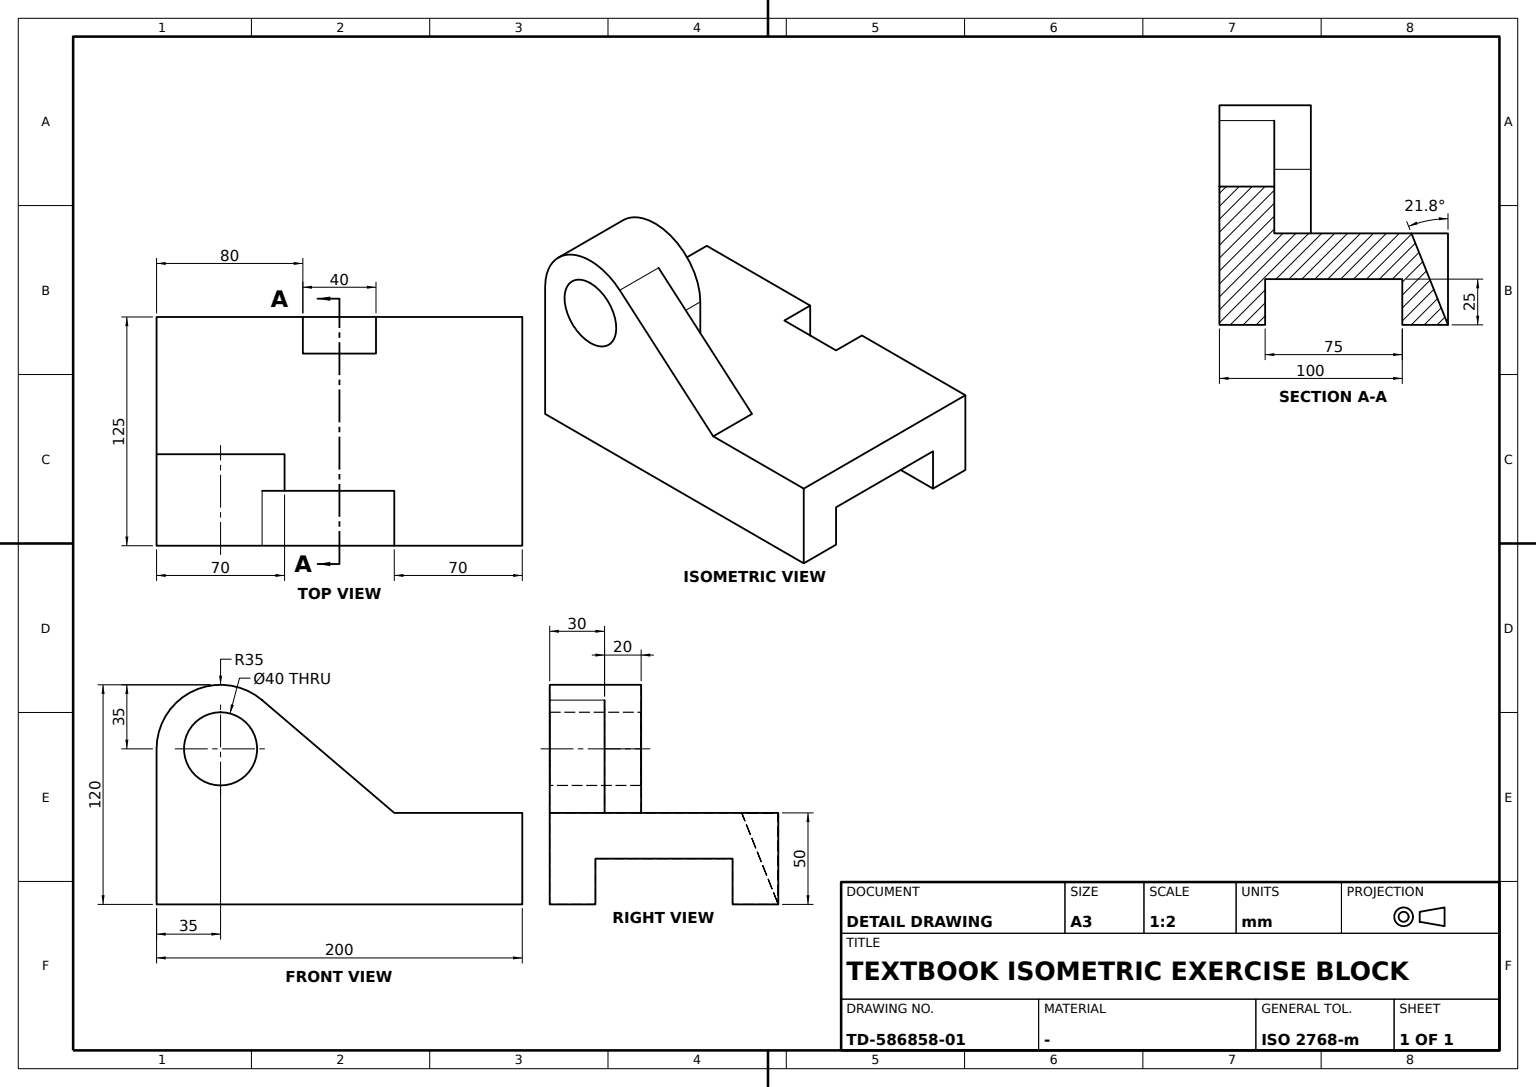
CATIA V5 part; units mm, degrees
sketch "Sketch1" plane through (0, 0, 0) normal (1, 0, 0) x (0, 1, 0)
  line L0 (-62.5, 50) -> (62.5, 50)
  line L1 (62.5, 50) -> (62.5, 0)
  point P0 (62.5, 0)
  line L2 (62.5, 0) -> (37.5, 0)
  line L3 (37.5, 0) -> (37.5, 25)
  line L4 (37.5, 25) -> (-37.5, 25)
  line L5 (-37.5, 25) -> (-37.5, 0)
  point P1 (-37.5, 0)
  line L6 (-37.5, 0) -> (-62.5, 0)
  line L7 (-62.5, 0) -> (-62.5, 50)
  dimension "length L4" = 75
  dimension "length L0" = 125
  dimension "length L5" = 25
  dimension "length L7" = 50
  constraint horizontal L0 x-axis
  constraint horizontal L2 x-axis
  constraint horizontal L4 x-axis
  constraint horizontal L6 x-axis
  constraint coincidence P0 x-axis
  constraint coincidence P1 x-axis
  constraint vertical L1 y-axis
  constraint vertical L3 y-axis
  constraint vertical L5 y-axis
  constraint vertical L7 y-axis
  constraint symmetry L7 L1 y-axis
  constraint symmetry L5 L3 y-axis
extrude "Pad1" add sketch "Sketch1" along normal mid plane 200
sketch "Sketch2" plane through (0, 0, 0) normal (1, 0, 0) x (0, 1, 0)
  line L0 (42.5, 50) -> (62.5, 0)
  point P0 (62.5, 0)
  line L1 (62.5, 0) -> (62.5, 50)
  line L2 (62.5, 50) -> (42.5, 50)
  line L3 (62.5, 0) -> (62.5, 50) construction
  line L4 (62.5, 50) -> (-62.5, 50) construction
  dimension "length L2" = 20
  dimension "distance L1 L3" = 0
  dimension "distance L2 L4" = 0
  constraint coincidence P0 x-axis
  constraint vertical L1 y-axis
  constraint horizontal L2 x-axis
extrude "Pocket1" cut sketch "Sketch2" along normal mid plane 40
sketch "Sketch3" plane through (0, -62.5, 0) normal (0, -1, 0) x (1, 0, 0)
  line L0 (-100, 50) -> (-30, 50)
  line L1 (-30, 50) -> (-30, 85)
  line L2 (-100, 85) -> (-100, 50)
  point P0 (-100, 85)
  line L3 (-100, 50) -> (100, 50) construction
  line L4 (-100, 50) -> (-100, 0) construction
  arc A0 (-30, 85) -> (-100, 85) centre (-65, 85) ccw
  circle A1 centre (-65, 85) radius 20
  dimension "distance L0 L3" = 0
  dimension "distance L4 L2" = 0
  dimension "radius A0" = 35
  dimension "length L1" = 35
  dimension "distance P0 L1" = 70
  dimension "radius A1" = 20
  constraint horizontal L0 x-axis
  constraint vertical L1 y-axis
  constraint vertical L2 y-axis
  constraint tangency A0 L0
extrude "Pad2" add sketch "Sketch3" against normal blind 50
sketch "Sketch4" plane through (0, -62.5, 0) normal (0, -1, 0) x (1, 0, 0)
  line L0 (-42.2927, 111.6341) -> (30, 50)
  point P0 (30, 50)
  line L1 (-30, 50) -> (-30, 85)
  point P1 (-30, 50)
  point P2 (-30, 85)
  line L2 (-30, 50) -> (100, 50) construction
  line L3 (-30, 50) -> (30, 50)
  point P3 (-30, 50)
  arc A0 (-30, 85) -> (-100, 85) centre (-65, 85) ccw construction
  arc A1 (-30, 85) -> (-42.2927, 111.6341) centre (-65, 85) ccw
  point P4 (-30, 85)
  line L4 (100, 50) -> (100, 0) construction
  point P5 (-42.2927, 111.6341)
  point P6 (-42.2927, 111.6341)
  dimension "distance P0 L4" = 70
  constraint tangency L0 A0
  constraint coincidence P0 L2
  constraint coincidence L0 P5
  constraint coincidence A0 P6
  constraint coincidence P1 P3
  constraint coincidence P2 P4
  constraint coincidence P5 P6
extrude "Pad3" add sketch "Sketch4" against normal blind 30
properties part number "13"
